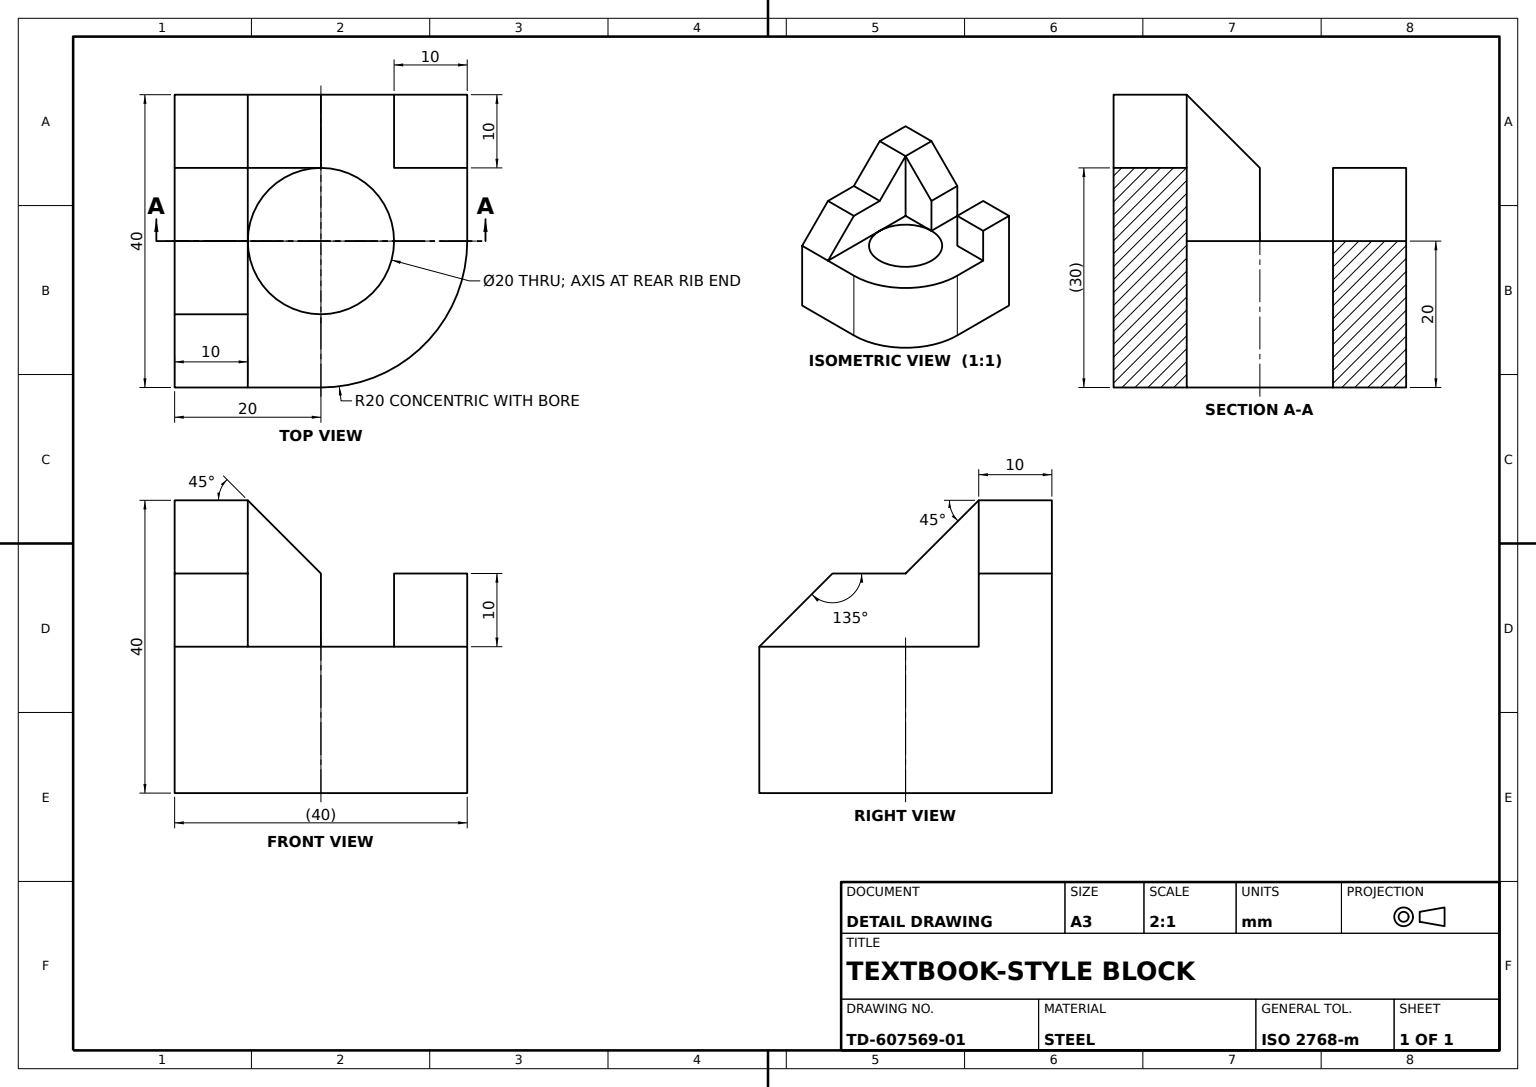
SolidWorks part; units mm, degrees
material "Plain Carbon Steel"
ref_plane "Front Plane" through (0, 0, 0) normal (0, 0, 1) x (1, 0, 0)
ref_plane "Top Plane" through (0, 0, 0) normal (0, 1, 0) x (1, 0, 0)
ref_plane "Right Plane" through (0, 0, 0) normal (1, 0, 0) x (0, 0, -1)
sketch "Base Block Profile" plane through (0, 0, 0) normal (0, 1, 0) x (1, 0, 0)
  line L1 (0, -20) -> (-20, -20)
  line L2 (20, 0) -> (20, 20)
  line L3 (20, 20) -> (-20, 20)
  line L4 (-20, -20) -> (-20, 20)
  line L5 (20, -20) -> (-20, 20) construction
  line L6 (20, 20) -> (-20, -20) construction
  arc A0 (0, -20) -> (20, 0) centre (0, 0) ccw
  point P0 (0, 0)
  dimension "D3" = 20
  dimension "D1" = 40
  dimension "D2" = 40
extrude "Base Block" add sketch "Base Block Profile" along normal mid plane 20
sketch "Corner Post Profile" plane through (0, 10, 0) normal (0, 1, 0) x (1, 0, 0)
  line L1 (20, 20) -> (10, 20)
  line L2 (20, 20) -> (20, 10)
  line L3 (20, 10) -> (10, 10)
  line L4 (10, 20) -> (10, 10)
  dimension "D1" = 10
  dimension "D2" = 10
extrude "Corner Post 10x10" add sketch "Corner Post Profile" along normal blind 10
sketch "Stepped Rib Profile" plane through (-20, 0, 0) normal (-1, 0, 0) x (0, 0, 1)
  line L0 (-20, 10) -> (-20, 30)
  line L1 (-20, 30) -> (-10, 30)
  line L2 (-10, 30) -> (0, 20)
  line L3 (0, 20) -> (10, 20)
  line L4 (10, 20) -> (20, 10)
  line L5 (-20, 20) -> (-10, 20) construction
  line L6 (-20, 10) -> (20, 10) construction
  line L7 (-20, 10) -> (20, 10)
  dimension "D1" = 10
  dimension "D2" = 10
  dimension "D3" = 10
  dimension "D4" = 20
extrude "Stepped Rib" add sketch "Stepped Rib Profile" against normal blind 10
sketch "Gusset Profile" plane through (0, 0, -20) normal (0, 0, -1) x (-1, 0, 0)
  line L0 (10, 30) -> (0, 20)
  line L1 (0, 20) -> (0, 10)
  line L2 (-10, 10) -> (10, 10) construction
  line L3 (-10, 10) -> (10, 10)
  line L4 (10, 30) -> (10, 10) construction
  line L5 (10, 30) -> (10, 10)
  line M4 (10, 30) -> (10, 10)
  line M5 (10, 10) -> (-10, 10)
  dimension "D1" = 10
extrude "Gusset" add sketch "Gusset Profile" against normal blind 10 contours L0 L1 M5 M4
sketch "Bore Profile" plane through (0, -10, 0) normal (0, -1, 0) x (1, 0, 0)
  circle A0 centre (0, 0) radius 10
  dimension "D1" = 20
extrude "Bore Ø20" cut sketch "Bore Profile" against normal up to surface (20 mm away) up to face at (4.9047, 10, -3.9842)
